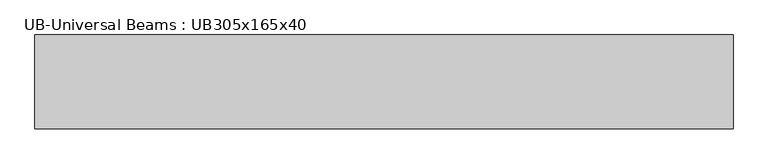
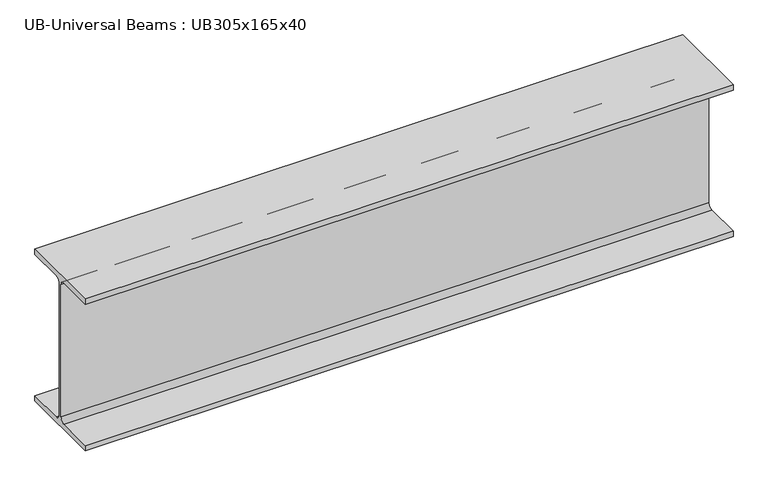
"""IFC4 building model written with IfcOpenShell, lengths in millimetres: beam geometry, UB-Universal Beams : UB305x165x40."""

from ifc_helpers import new_model, si_unit, point, frame, frame_2d, origin, place, context, project, spatial, polyline, circle_curve, trimmed, segment, composite_curve, outline, extrude, source, transform, mapped, element, save


def ub_universal_beams_ub305x165x40_ef0a91e2(model_context):
    return source(origin(), model_context, "Body", "SweptSolid", [
        extrude(outline(composite_curve([segment(polyline([(82.5, -141.5), (82.5, -151.7), (-82.5, -151.7), (-82.5, -141.5), (-11.9, -141.5)]), True, "CONTINUOUS"), segment(trimmed(circle_curve(frame_2d((-11.9, -132.6)), 8.9), [point((-11.9, -141.5))], [point((-3.0, -132.6))], True, "CARTESIAN"), True, "CONTINUOUS"), segment(polyline([(-3.0, -132.6), (-3.0, 132.6)]), True, "CONTINUOUS"), segment(trimmed(circle_curve(frame_2d((-11.9, 132.6)), 8.9), [point((-3.0, 132.6))], [point((-11.9, 141.5))], True, "CARTESIAN"), True, "CONTINUOUS"), segment(polyline([(-11.9, 141.5), (-82.5, 141.5), (-82.5, 151.7), (82.5, 151.7), (82.5, 141.5), (11.9, 141.5)]), True, "CONTINUOUS"), segment(trimmed(circle_curve(frame_2d((11.9, 132.6)), 8.9), [point((11.9, 141.5))], [point((3.0, 132.6))], True, "CARTESIAN"), True, "CONTINUOUS"), segment(polyline([(3.0, 132.6), (3.0, -132.6)]), True, "CONTINUOUS"), segment(trimmed(circle_curve(frame_2d((11.9, -132.6)), 8.9), [point((3.0, -132.6))], [point((11.9, -141.5))], True, "CARTESIAN"), True, "CONTINUOUS"), segment(polyline([(11.9, -141.5), (82.5, -141.5)]), True, "CONTINUOUS")], self_intersect=False)), frame((-625.85, 0.0, 0.0), z_axis=(1.0, 0.0, 0.0), x_axis=(0.0, 1.0, 0.0)), (0.0, 0.0, 1.0), 1225.9),
    ])


if __name__ == "__main__":
    model = new_model("IFC4")
    model_context = context("Model", 3, world=origin())
    ifc_project = project(units=[si_unit("LENGTHUNIT", "METRE", prefix="MILLI")], contexts=[model_context])
    site = spatial("IfcSite", under=ifc_project)
    building = spatial("IfcBuilding", under=site)
    placement = place(None, origin())
    ub_universal_beams_ub305x165x40_shape = ub_universal_beams_ub305x165x40_ef0a91e2(model_context)
    element("IfcBeam", 1, ObjectType="UB-Universal Beams : UB305x165x40", at=placement, inside=building, context=model_context, shape_type="MappedRepresentation", body=[
        mapped(ub_universal_beams_ub305x165x40_shape, transform((0.0, 0.0, 0.0), x_axis=(1.0, 0.0, 0.0), y_axis=(0.0, 1.0, 0.0), z_axis=(0.0, 0.0, 1.0))),
    ])
    save(model, "model.ifc")

# Revit data of these elements
# Type "UB-Universal Beams : UB305x165x40"
#   Section Name Key = "UB305X165X40"
#   Width = 16.5 cm
#   Web Thickness = 0.6 cm
#   Web Fillet = 0.89 cm
#   Warping Constant = 164000.0 cm⁶
#   Torsional Moment of Inertia = 14.70 cm⁴
#   Section Area = 51.3 cm²
#   Plastic Modulus weak axis = 142.0 cm³
#   Plastic Modulus strong axis = 623.0 cm³
#   Nominal Weight = 40.2999 kgf/m
#   Moment of Inertia weak axis = 764.00 cm⁴
#   Moment of Inertia strong axis = 8503.00 cm⁴
#   Height = 30.34 cm
#   Flange Thickness = 1.02 cm
#   Elastic Modulus weak axis = 92.6 cm³
#   Elastic Modulus strong axis = 560.0 cm³
#   Centroid Vertical = 15.17 cm
#   Centroid Horizontal = 8.25 cm
#   Bolt Spacing = 9.0 cm
#   Length [instance default] = 1500 mm
#   Structural Material [instance default] = Metal - Steel 43-275
#   Type Comments = ""
#   Assembly Code = ""
# Element 1 (IfcBeam, "UB-Universal Beams : UB305x165x40")
#   Materials on its faces: "Metal - Steel 43-275"
# Materials
#   "Metal - Steel 43-275": class "Metal", colour RGB 247 247 247, transparency 0, Cost = 0
